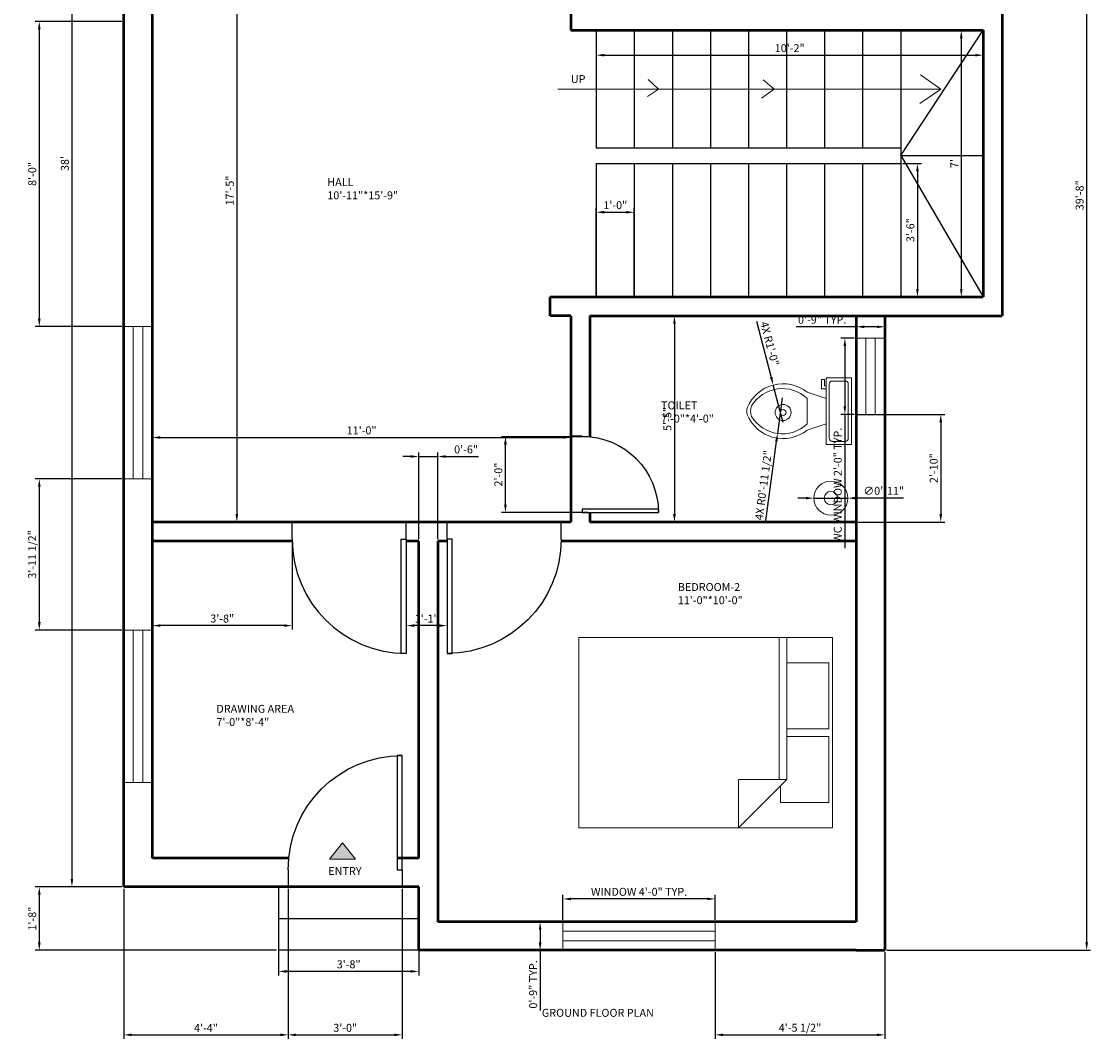
# Model space of a CAD drawing. Units: inches. Extents: x 1994 to 2331, y 1752 to 2286.
# Tile 1 of 2: x 1994 to 2331, y 1752 to 2073. Entities that reach past the tile are written whole.
import ezdxf

# ---------------------------------------------------------------- set-up
doc = ezdxf.new("R2010")
doc.units = ezdxf.units.IN
for name, color, linetype, lineweight in [('A-ANNO-DIMS', 2, 'Continuous', 18), ('A-ANNO-PATT', 7, 'Continuous', 18), ('A-ANNO-SYMB', 7, 'Continuous', 18), ('A-ANNO-TEXT', 7, 'Continuous', 25), ('A-AREA-IDEN', 7, 'Continuous', 25), ('A-DOOR', 3, 'Continuous', 25), ('A-FLOR-FIXT', 8, 'Continuous', 18), ('A-FLOR-STRS', 7, 'Continuous', 25), ('A-FURN', 9, 'Continuous', 18), ('A-GLAZ', 4, 'Continuous', 18), ('A-WALL', 7, 'Continuous', 50)]:
    doc.layers.add(name, color=color, linetype=linetype, lineweight=lineweight)
doc.styles.get("Standard").update_dxf_attribs({"font": 'arial.ttf'})
doc.dimstyles.new('ISO-25', dxfattribs={"dimtxt": 2.5, "dimasz": 2.5, "dimexe": 1.25, "dimexo": 0.625, "dimtad": 1, "dimdec": 1, "dimlunit": 3, "dimtxsty": 'Standard', "dimcen": 2.5, "dimadec": 0, "dimazin": 0, "dimtfac": 1, "dimtdec": 1, "dimtmove": 0, "dimatfit": 3, "dimfxl": 1, "dimarcsym": 0})

# ---------------------------------------------------------------- blocks, each defined once
blk = doc.blocks.new('*U2')
for p, q in [((0, 0), (0, -6)), ((40, 0), (40, -6))]:
    blk.add_line(p, q)
blk.add_lwpolyline([(0, 0), (0, 40), (1.75, 40), (1.75, 0)], close=True)
blk.add_arc((0, 0), 40, 0, 90)
blk = doc.blocks.new('Bed - Queen')
for p, q in [((0, -80.00003), (0, 0)), ((0, 0), (59.99999, 0)), ((59.99999, 0), (59.99999, -80.00003)), ((7.99999, -1.2), (28.79998, -1.2)), ((7.99999, -14.4), (7.99999, -1.2)), ((28.79998, -1.2), (28.79998, -14.4)), ((31.19999, -1.2), (51.99999, -1.2)), ((31.19999, -14.4), (31.19999, -1.2)), ((51.99999, -1.2), (51.99999, -16.4)), ((0, -14.4), (44.8, -14.4)), ((44.8, -16.8), (0, -16.8)), ((59.99999, -29.6), (44.8, -14.4)), ((44.8, -14.4), (44.8, -29.6)), ((51.99999, -16.4), (46.79936, -16.4)), ((44.8, -29.6), (59.99999, -29.6)), ((59.99999, -80.00003), (0, -80.00003))]:
    blk.add_line(p, q)
blk = doc.blocks.new('Toilet - top')
for p, q in [((9.5, -6), (9.5, -2)), ((-10, -8.5), (-8, -8.5)), ((-10, -9.5), (-10, -8.5)), ((-7, -9.5), (-10, -9.5)), ((-8, -8.5), (-8, -8)), ((-7, -8), (-7, -9.5)), ((-4, -8), (-6, -14)), ((4, -8), (6, -14)), ((4, -14), (-4, -14))]:
    blk.add_line(p, q)
blk.add_lwpolyline([(10.5, -8), (10.5, 0), (-10.5, 0), (-10.5, -8)], close=True)
for points in [[(-9.5, -2), (-9.5, -6)], [(8.5, -1), (-8.5, -1)], [(-8.5, -7), (8.5, -7)]]:
    blk.add_lwpolyline(points)
for centre, radius, start, end in [((-8.62, -1.88), 0.884, 81.8699, 188.1301), ((8.62, -1.88), 0.884, 351.8699, 98.1301), ((-8.62, -6.12), 0.884, 171.8699, 278.1301), ((8.62, -6.12), 0.884, 261.8699, 8.1301), ((3.52, -21.58), 12.17, 141.4691, 247.9714), ((4.2, -21.82), 11.33, 136.3677, 238.9468), ((-3.52, -21.58), 12.17, 292.0284, 38.5307), ((-4.2, -21.82), 11.33, 301.053, 43.6321), ((0, -27.88), 4, 245.7318, 294.2682), ((0, -29), 4, 254.8605, 285.1395)]:
    blk.add_arc(centre, radius, start, end)
blk = doc.blocks.new('*D7')
at = {"layer": 'A-ANNO-DIMS', "color": 0, "lineweight": -2, "transparency": 16777216}
for p, q in [((2025.95, 2256.2), (2008.97, 2256.2)), ((2010.22, 2253.7), (2010.22, 1802.7)), ((2025.95, 1800.2), (2008.97, 1800.2))]:
    blk.add_line(p, q, dxfattribs=at)
at = {"layer": 'A-ANNO-DIMS', "color": 0, "transparency": 16777216}
for points in [[(2009.8, 2253.7), (2010.63, 2253.7), (2010.22, 2256.2)], [(2009.8, 1802.7), (2010.63, 1802.7), (2010.22, 1800.2)]]:
    blk.add_solid(points, dxfattribs=at)
at = {"layer": 'Defpoints', "color": 0, "transparency": 16777216}
for p in [(2026.58, 2256.2), (2010.22, 1800.2), (2026.58, 1800.2)]:
    blk.add_point(p, dxfattribs=at)
at = {"layer": 'A-ANNO-DIMS', "color": 0, "transparency": 16777216, "insert": (2008.31, 2028.2), "char_height": 2.5, "attachment_point": 5, "rotation": 90}
blk.add_mtext("38'", dxfattribs=at)
blk = doc.blocks.new('*D9')
at = {"layer": 'A-ANNO-DIMS', "color": 0, "lineweight": -2, "transparency": 16777216}
for p, q in [((2296.95, 2070.2), (2289.44, 2070.2)), ((2290.69, 2067.7), (2290.69, 1988.7)), ((2296.95, 1986.2), (2289.44, 1986.2))]:
    blk.add_line(p, q, dxfattribs=at)
at = {"layer": 'A-ANNO-DIMS', "color": 0, "transparency": 16777216}
for points in [[(2290.28, 2067.7), (2291.11, 2067.7), (2290.69, 2070.2)], [(2290.28, 1988.7), (2291.11, 1988.7), (2290.69, 1986.2)]]:
    blk.add_solid(points, dxfattribs=at)
at = {"layer": 'Defpoints', "color": 0, "transparency": 16777216}
for p in [(2297.58, 2070.2), (2290.69, 1986.2), (2297.58, 1986.2)]:
    blk.add_point(p, dxfattribs=at)
at = {"layer": 'A-ANNO-DIMS', "color": 0, "transparency": 16777216, "insert": (2288.82, 2028.2), "char_height": 2.5, "attachment_point": 5, "rotation": 90}
blk.add_mtext("7'", dxfattribs=at)
blk = doc.blocks.new('*D10')
at = {"layer": 'A-ANNO-DIMS', "color": 0, "lineweight": -2, "transparency": 16777216}
for p, q in [((2272.2, 2028.2), (2278.11, 2028.2)), ((2276.86, 2025.7), (2276.86, 1988.7)), ((2272.2, 1986.2), (2278.11, 1986.2))]:
    blk.add_line(p, q, dxfattribs=at)
at = {"layer": 'A-ANNO-DIMS', "color": 0, "transparency": 16777216}
for points in [[(2276.44, 2025.7), (2277.28, 2025.7), (2276.86, 2028.2)], [(2276.44, 1988.7), (2277.28, 1988.7), (2276.86, 1986.2)]]:
    blk.add_solid(points, dxfattribs=at)
at = {"layer": 'Defpoints', "color": 0, "transparency": 16777216}
for p in [(2271.58, 2028.2), (2271.58, 1986.2), (2276.86, 1986.2)]:
    blk.add_point(p, dxfattribs=at)
at = {"layer": 'A-ANNO-DIMS', "color": 0, "transparency": 16777216, "insert": (2274.96, 2007.2), "char_height": 2.5, "attachment_point": 5, "rotation": 90}
blk.add_mtext('3\'-6"', dxfattribs=at)
blk = doc.blocks.new('*D11')
at = {"layer": 'A-ANNO-DIMS', "color": 0, "lineweight": -2, "transparency": 16777216}
for p, q in [((2175.58, 2069.58), (2175.58, 2061.11)), ((2297.58, 2069.58), (2297.58, 2061.11)), ((2178.08, 2062.36), (2295.08, 2062.36))]:
    blk.add_line(p, q, dxfattribs=at)
at = {"layer": 'A-ANNO-DIMS', "color": 0, "transparency": 16777216}
for points in [[(2178.08, 2062.78), (2178.08, 2061.95), (2175.58, 2062.36)], [(2295.08, 2062.78), (2295.08, 2061.95), (2297.58, 2062.36)]]:
    blk.add_solid(points, dxfattribs=at)
at = {"layer": 'Defpoints', "color": 0, "transparency": 16777216}
for p in [(2175.58, 2070.2), (2297.58, 2070.2), (2297.58, 2062.36)]:
    blk.add_point(p, dxfattribs=at)
at = {"layer": 'A-ANNO-DIMS', "color": 0, "transparency": 16777216, "insert": (2236.58, 2064.26), "char_height": 2.5, "attachment_point": 5}
blk.add_mtext('10\'-2"', dxfattribs=at)
blk = doc.blocks.new('WIN-48IN')
for p, q in [((0, 9), (48, 9)), ((0, 0), (0, 9)), ((48, 9), (48, 0)), ((0, 6), (48, 6)), ((48, 3), (0, 3)), ((48, 0), (0, 0))]:
    blk.add_line(p, q)
blk = doc.blocks.new('WIN-24IN')
for p, q in [((0, 0), (0, 24)), ((0, 24), (9, 24)), ((3, 0), (3, 24)), ((6, 24), (6, 0)), ((9, 24), (9, 0)), ((9, 0), (0, 0))]:
    blk.add_line(p, q)
blk = doc.blocks.new('*D14')
at = {"layer": 'A-ANNO-DIMS', "color": 0, "lineweight": -2, "transparency": 16777216}
for p, q in [((2165.08, 1789.83), (2165.08, 1797.65)), ((2213.08, 1789.83), (2213.08, 1797.65)), ((2210.58, 1796.4), (2167.58, 1796.4))]:
    blk.add_line(p, q, dxfattribs=at)
at = {"layer": 'A-ANNO-DIMS', "color": 0, "transparency": 16777216}
for points in [[(2167.58, 1796.82), (2167.58, 1795.99), (2165.08, 1796.4)], [(2210.58, 1796.82), (2210.58, 1795.99), (2213.08, 1796.4)]]:
    blk.add_solid(points, dxfattribs=at)
at = {"layer": 'Defpoints', "color": 0, "transparency": 16777216}
for p in [(2165.08, 1796.4), (2165.08, 1789.2), (2213.08, 1789.2)]:
    blk.add_point(p, dxfattribs=at)
at = {"layer": 'A-ANNO-DIMS', "color": 0, "transparency": 16777216, "insert": (2189.08, 1798.32), "char_height": 2.5, "attachment_point": 5}
blk.add_mtext('WINDOW 4\'-0" TYP.', dxfattribs=at)
blk = doc.blocks.new('*D15')
at = {"layer": 'A-ANNO-DIMS', "color": 0, "lineweight": -2, "transparency": 16777216}
for p, q in [((2164.46, 1789.2), (2156.63, 1789.2)), ((2157.88, 1786.7), (2157.88, 1782.7)), ((2164.46, 1780.2), (2156.63, 1780.2)), ((2157.88, 1780.2), (2157.88, 1761.22))]:
    blk.add_line(p, q, dxfattribs=at)
at = {"layer": 'A-ANNO-DIMS', "color": 0, "transparency": 16777216}
for points in [[(2157.46, 1786.7), (2158.3, 1786.7), (2157.88, 1789.2)], [(2157.46, 1782.7), (2158.3, 1782.7), (2157.88, 1780.2)]]:
    blk.add_solid(points, dxfattribs=at)
at = {"layer": 'Defpoints', "color": 0, "transparency": 16777216}
for p in [(2165.08, 1789.2), (2157.88, 1780.2), (2165.08, 1780.2)]:
    blk.add_point(p, dxfattribs=at)
at = {"layer": 'A-ANNO-DIMS', "color": 0, "transparency": 16777216, "insert": (2155.98, 1769.46), "char_height": 2.5, "attachment_point": 5, "rotation": 90}
blk.add_mtext('0\'-9" TYP.', dxfattribs=at)
blk = doc.blocks.new('*D16')
at = {"layer": 'A-ANNO-DIMS', "color": 0, "lineweight": -2, "transparency": 16777216}
for p, q in [((2256.95, 1973.15), (2252.73, 1973.15)), ((2253.98, 1970.65), (2253.98, 1951.65)), ((2256.95, 1949.15), (2252.73, 1949.15)), ((2253.98, 1949.15), (2253.98, 1906.97))]:
    blk.add_line(p, q, dxfattribs=at)
at = {"layer": 'A-ANNO-DIMS', "color": 0, "transparency": 16777216}
for points in [[(2253.56, 1970.65), (2254.4, 1970.65), (2253.98, 1973.15)], [(2253.56, 1951.65), (2254.4, 1951.65), (2253.98, 1949.15)]]:
    blk.add_solid(points, dxfattribs=at)
at = {"layer": 'Defpoints', "color": 0, "transparency": 16777216}
for p in [(2257.58, 1973.15), (2253.98, 1949.15), (2257.58, 1949.15)]:
    blk.add_point(p, dxfattribs=at)
at = {"layer": 'A-ANNO-DIMS', "color": 0, "transparency": 16777216, "insert": (2252.06, 1926.81), "char_height": 2.5, "attachment_point": 5, "rotation": 90}
blk.add_mtext('WC WINDOW 2\'-0" TYP.', dxfattribs=at)
blk = doc.blocks.new('*D17')
at = {"layer": 'A-ANNO-DIMS', "color": 0, "lineweight": -2, "transparency": 16777216}
for p, q in [((2257.58, 1976.75), (2238.59, 1976.75)), ((2257.58, 1973.77), (2257.58, 1978)), ((2264.08, 1976.75), (2260.08, 1976.75)), ((2266.58, 1973.77), (2266.58, 1978))]:
    blk.add_line(p, q, dxfattribs=at)
at = {"layer": 'A-ANNO-DIMS', "color": 0, "transparency": 16777216}
for points in [[(2260.08, 1977.16), (2260.08, 1976.33), (2257.58, 1976.75)], [(2264.08, 1977.16), (2264.08, 1976.33), (2266.58, 1976.75)]]:
    blk.add_solid(points, dxfattribs=at)
at = {"layer": 'Defpoints', "color": 0, "transparency": 16777216}
for p in [(2257.58, 1976.75), (2257.58, 1973.15), (2266.58, 1973.15)]:
    blk.add_point(p, dxfattribs=at)
at = {"layer": 'A-ANNO-DIMS', "color": 0, "transparency": 16777216, "insert": (2246.83, 1978.65), "char_height": 2.5, "attachment_point": 5}
blk.add_mtext('0\'-9" TYP.', dxfattribs=at)
blk = doc.blocks.new('*D24')
at = {"layer": 'A-ANNO-DIMS', "color": 0, "lineweight": -2, "transparency": 16777216}
for p, q in [((2267.2, 2256.2), (2331.48, 2256.2)), ((2330.23, 2253.7), (2330.23, 1782.7)), ((2267.2, 1780.2), (2331.48, 1780.2))]:
    blk.add_line(p, q, dxfattribs=at)
at = {"layer": 'A-ANNO-DIMS', "color": 0, "transparency": 16777216}
for points in [[(2329.81, 2253.7), (2330.65, 2253.7), (2330.23, 2256.2)], [(2329.81, 1782.7), (2330.65, 1782.7), (2330.23, 1780.2)]]:
    blk.add_solid(points, dxfattribs=at)
at = {"layer": 'Defpoints', "color": 0, "transparency": 16777216}
for p in [(2266.58, 2256.2), (2266.58, 1780.2), (2330.23, 1780.2)]:
    blk.add_point(p, dxfattribs=at)
at = {"layer": 'A-ANNO-DIMS', "color": 0, "transparency": 16777216, "insert": (2328.33, 2018.2), "char_height": 2.5, "attachment_point": 5, "rotation": 90}
blk.add_mtext('39\'-8"', dxfattribs=at)
blk = doc.blocks.new('*D26')
at = {"layer": 'A-ANNO-DIMS', "color": 0, "lineweight": -2, "transparency": 16777216}
for p, q in [((2025.95, 1800.2), (1998.68, 1800.2)), ((1999.93, 1797.7), (1999.93, 1782.7)), ((2074.77, 1780.2), (1998.68, 1780.2))]:
    blk.add_line(p, q, dxfattribs=at)
at = {"layer": 'A-ANNO-DIMS', "color": 0, "transparency": 16777216}
for points in [[(1999.51, 1797.7), (2000.35, 1797.7), (1999.93, 1800.2)], [(1999.51, 1782.7), (2000.35, 1782.7), (1999.93, 1780.2)]]:
    blk.add_solid(points, dxfattribs=at)
at = {"layer": 'Defpoints', "color": 0, "transparency": 16777216}
for p in [(2026.58, 1800.2), (1999.93, 1780.2), (2075.4, 1780.2)]:
    blk.add_point(p, dxfattribs=at)
at = {"layer": 'A-ANNO-DIMS', "color": 0, "transparency": 16777216, "insert": (1998.03, 1790.2), "char_height": 2.5, "attachment_point": 5, "rotation": 90}
blk.add_mtext('1\'-8"', dxfattribs=at)
blk = doc.blocks.new('*D30')
at = {"layer": 'A-ANNO-DIMS', "color": 0, "lineweight": -2, "transparency": 16777216}
for p, q in [((2025.95, 2073.01), (1998.68, 2073.01)), ((1999.93, 2070.51), (1999.93, 1979.32)), ((2025.95, 1976.82), (1998.68, 1976.82))]:
    blk.add_line(p, q, dxfattribs=at)
at = {"layer": 'A-ANNO-DIMS', "color": 0, "transparency": 16777216}
for points in [[(1999.51, 2070.51), (2000.35, 2070.51), (1999.93, 2073.01)], [(1999.51, 1979.32), (2000.35, 1979.32), (1999.93, 1976.82)]]:
    blk.add_solid(points, dxfattribs=at)
at = {"layer": 'Defpoints', "color": 0, "transparency": 16777216}
for p in [(2026.58, 2073.01), (1999.93, 1976.82), (2026.58, 1976.82)]:
    blk.add_point(p, dxfattribs=at)
at = {"layer": 'A-ANNO-DIMS', "color": 0, "transparency": 16777216, "insert": (1998.03, 2024.91), "char_height": 2.5, "attachment_point": 5, "rotation": 90}
blk.add_mtext('8\'-0"', dxfattribs=at)
blk = doc.blocks.new('*D31')
at = {"layer": 'A-ANNO-DIMS', "color": 0, "lineweight": -2, "transparency": 16777216}
for p, q in [((2025.95, 1928.82), (1998.68, 1928.82)), ((1999.93, 1926.32), (1999.93, 1883.65)), ((2025.95, 1881.15), (1998.68, 1881.15))]:
    blk.add_line(p, q, dxfattribs=at)
at = {"layer": 'A-ANNO-DIMS', "color": 0, "transparency": 16777216}
for points in [[(1999.51, 1926.32), (2000.35, 1926.32), (1999.93, 1928.82)], [(1999.51, 1883.65), (2000.35, 1883.65), (1999.93, 1881.15)]]:
    blk.add_solid(points, dxfattribs=at)
at = {"layer": 'Defpoints', "color": 0, "transparency": 16777216}
for p in [(2026.58, 1928.82), (1999.93, 1881.15), (2026.58, 1881.15)]:
    blk.add_point(p, dxfattribs=at)
at = {"layer": 'A-ANNO-DIMS', "color": 0, "transparency": 16777216, "insert": (1998.01, 1904.99), "char_height": 2.5, "attachment_point": 5, "rotation": 90}
blk.add_mtext('3\'-11 1/2"', dxfattribs=at)
blk = doc.blocks.new('*D34')
at = {"layer": 'A-ANNO-DIMS', "color": 0, "lineweight": -2, "transparency": 16777216}
for p, q in [((2258.2, 1949.15), (2285.48, 1949.15)), ((2284.23, 1946.65), (2284.23, 1917.7)), ((2258.2, 1915.2), (2285.48, 1915.2))]:
    blk.add_line(p, q, dxfattribs=at)
at = {"layer": 'A-ANNO-DIMS', "color": 0, "transparency": 16777216}
for points in [[(2283.81, 1946.65), (2284.65, 1946.65), (2284.23, 1949.15)], [(2283.81, 1917.7), (2284.65, 1917.7), (2284.23, 1915.2)]]:
    blk.add_solid(points, dxfattribs=at)
at = {"layer": 'Defpoints', "color": 0, "transparency": 16777216}
for p in [(2257.58, 1949.15), (2257.58, 1915.2), (2284.23, 1915.2)]:
    blk.add_point(p, dxfattribs=at)
at = {"layer": 'A-ANNO-DIMS', "color": 0, "transparency": 16777216, "insert": (2282.33, 1932.18), "char_height": 2.5, "attachment_point": 5, "rotation": 90}
blk.add_mtext('2\'-10"', dxfattribs=at)
blk = doc.blocks.new('*D35')
at = {"layer": 'A-ANNO-DIMS', "color": 0, "lineweight": -2, "transparency": 16777216}
for p, q in [((2213.08, 1779.58), (2213.08, 1752.3)), ((2266.58, 1779.58), (2266.58, 1752.3)), ((2215.58, 1753.55), (2264.08, 1753.55))]:
    blk.add_line(p, q, dxfattribs=at)
at = {"layer": 'A-ANNO-DIMS', "color": 0, "transparency": 16777216}
for points in [[(2215.58, 1753.97), (2215.58, 1753.14), (2213.08, 1753.55)], [(2264.08, 1753.97), (2264.08, 1753.14), (2266.58, 1753.55)]]:
    blk.add_solid(points, dxfattribs=at)
at = {"layer": 'Defpoints', "color": 0, "transparency": 16777216}
for p in [(2213.08, 1780.2), (2266.58, 1780.2), (2266.58, 1753.55)]:
    blk.add_point(p, dxfattribs=at)
at = {"layer": 'A-ANNO-DIMS', "color": 0, "transparency": 16777216, "insert": (2239.83, 1755.47), "char_height": 2.5, "attachment_point": 5}
blk.add_mtext('4\'-5 1/2"', dxfattribs=at)
blk = doc.blocks.new('*D36')
at = {"layer": 'A-ANNO-DIMS', "color": 0, "lineweight": -2, "transparency": 16777216}
for p, q in [((2174.2, 1980.2), (2201.48, 1980.2)), ((2200.23, 1977.7), (2200.23, 1917.7)), ((2174.2, 1915.2), (2201.48, 1915.2))]:
    blk.add_line(p, q, dxfattribs=at)
at = {"layer": 'A-ANNO-DIMS', "color": 0, "transparency": 16777216}
for points in [[(2199.81, 1977.7), (2200.65, 1977.7), (2200.23, 1980.2)], [(2199.81, 1917.7), (2200.65, 1917.7), (2200.23, 1915.2)]]:
    blk.add_solid(points, dxfattribs=at)
at = {"layer": 'Defpoints', "color": 0, "transparency": 16777216}
for p in [(2173.58, 1980.2), (2173.58, 1915.2), (2200.23, 1915.2)]:
    blk.add_point(p, dxfattribs=at)
at = {"layer": 'A-ANNO-DIMS', "color": 0, "transparency": 16777216, "insert": (2198.33, 1947.7), "char_height": 2.5, "attachment_point": 5, "rotation": 90}
blk.add_mtext('5\'-5"', dxfattribs=at)
blk = doc.blocks.new('*D37')
at = {"layer": 'A-ANNO-DIMS', "color": 0, "lineweight": -2, "transparency": 16777216}
for p, q in [((2175.58, 1986.83), (2175.58, 2014.1)), ((2187.58, 1986.83), (2187.58, 2014.1)), ((2178.08, 2012.85), (2185.08, 2012.85))]:
    blk.add_line(p, q, dxfattribs=at)
at = {"layer": 'A-ANNO-DIMS', "color": 0, "transparency": 16777216}
for points in [[(2178.08, 2013.27), (2178.08, 2012.44), (2175.58, 2012.85)], [(2185.08, 2013.27), (2185.08, 2012.44), (2187.58, 2012.85)]]:
    blk.add_solid(points, dxfattribs=at)
at = {"layer": 'Defpoints', "color": 0, "transparency": 16777216}
for p in [(2187.58, 2012.85), (2175.58, 1986.2), (2187.58, 1986.2)]:
    blk.add_point(p, dxfattribs=at)
at = {"layer": 'A-ANNO-DIMS', "color": 0, "transparency": 16777216, "insert": (2181.58, 2014.76), "char_height": 2.5, "attachment_point": 5}
blk.add_mtext('1\'-0"', dxfattribs=at)
blk = doc.blocks.new('*D38')
at = {"layer": 'A-ANNO-DIMS', "color": 0, "lineweight": -2, "transparency": 16777216}
for p, q in [((2117.08, 1935.85), (2114.58, 1935.85)), ((2119.58, 1909.83), (2119.58, 1937.1)), ((2119.58, 1935.85), (2125.58, 1935.85)), ((2125.58, 1909.83), (2125.58, 1937.1)), ((2128.08, 1935.85), (2138.47, 1935.85))]:
    blk.add_line(p, q, dxfattribs=at)
at = {"layer": 'A-ANNO-DIMS', "color": 0, "transparency": 16777216}
for points in [[(2117.08, 1936.27), (2117.08, 1935.44), (2119.58, 1935.85)], [(2128.08, 1936.27), (2128.08, 1935.44), (2125.58, 1935.85)]]:
    blk.add_solid(points, dxfattribs=at)
at = {"layer": 'Defpoints', "color": 0, "transparency": 16777216}
for p in [(2125.58, 1935.85), (2119.58, 1909.2), (2125.58, 1909.2)]:
    blk.add_point(p, dxfattribs=at)
at = {"layer": 'A-ANNO-DIMS', "color": 0, "transparency": 16777216, "insert": (2134.53, 1937.76), "char_height": 2.5, "attachment_point": 5}
blk.add_mtext('0\'-6"', dxfattribs=at)
blk = doc.blocks.new('*D39')
at = {"layer": 'A-ANNO-DIMS', "color": 0, "lineweight": -2, "transparency": 16777216}
for p, q in [((2026.58, 1799.58), (2026.58, 1752.3)), ((2078.4, 1799.58), (2078.4, 1752.3)), ((2029.08, 1753.55), (2075.9, 1753.55))]:
    blk.add_line(p, q, dxfattribs=at)
at = {"layer": 'A-ANNO-DIMS', "color": 0, "transparency": 16777216}
for points in [[(2029.08, 1753.97), (2029.08, 1753.14), (2026.58, 1753.55)], [(2075.9, 1753.97), (2075.9, 1753.14), (2078.4, 1753.55)]]:
    blk.add_solid(points, dxfattribs=at)
at = {"layer": 'Defpoints', "color": 0, "transparency": 16777216}
for p in [(2026.58, 1800.2), (2078.4, 1800.2), (2078.4, 1753.55)]:
    blk.add_point(p, dxfattribs=at)
at = {"layer": 'A-ANNO-DIMS', "color": 0, "transparency": 16777216, "insert": (2052.49, 1755.43), "char_height": 2.5, "attachment_point": 5}
blk.add_mtext('4\'-4"', dxfattribs=at)
blk = doc.blocks.new('*D40')
at = {"layer": 'A-ANNO-DIMS', "color": 0, "lineweight": -2, "transparency": 16777216}
for p, q in [((2036.2, 2124.2), (2063.48, 2124.2)), ((2062.23, 2121.7), (2062.23, 1917.7)), ((2036.2, 1915.2), (2063.48, 1915.2))]:
    blk.add_line(p, q, dxfattribs=at)
at = {"layer": 'A-ANNO-DIMS', "color": 0, "transparency": 16777216}
for points in [[(2061.81, 2121.7), (2062.65, 2121.7), (2062.23, 2124.2)], [(2061.81, 1917.7), (2062.65, 1917.7), (2062.23, 1915.2)]]:
    blk.add_solid(points, dxfattribs=at)
at = {"layer": 'Defpoints', "color": 0, "transparency": 16777216}
for p in [(2035.58, 2124.2), (2035.58, 1915.2), (2062.23, 1915.2)]:
    blk.add_point(p, dxfattribs=at)
at = {"layer": 'A-ANNO-DIMS', "color": 0, "transparency": 16777216, "insert": (2060.33, 2019.7), "char_height": 2.5, "attachment_point": 5, "rotation": 90}
blk.add_mtext('17\'-5"', dxfattribs=at)
blk = doc.blocks.new('*D41')
at = {"layer": 'A-ANNO-DIMS', "color": 0, "lineweight": -2, "transparency": 16777216}
for p, q in [((2035.58, 1915.83), (2035.58, 1943.1)), ((2167.58, 1915.83), (2167.58, 1943.1)), ((2038.08, 1941.85), (2165.08, 1941.85))]:
    blk.add_line(p, q, dxfattribs=at)
at = {"layer": 'A-ANNO-DIMS', "color": 0, "transparency": 16777216}
for points in [[(2038.08, 1942.27), (2038.08, 1941.44), (2035.58, 1941.85)], [(2165.08, 1942.27), (2165.08, 1941.44), (2167.58, 1941.85)]]:
    blk.add_solid(points, dxfattribs=at)
at = {"layer": 'Defpoints', "color": 0, "transparency": 16777216}
for p in [(2167.58, 1941.85), (2035.58, 1915.2), (2167.58, 1915.2)]:
    blk.add_point(p, dxfattribs=at)
at = {"layer": 'A-ANNO-DIMS', "color": 0, "transparency": 16777216, "insert": (2101.58, 1943.76), "char_height": 2.5, "attachment_point": 5}
blk.add_mtext('11\'-0"', dxfattribs=at)
blk = doc.blocks.new('*D42')
at = {"layer": 'A-ANNO-DIMS', "color": 0, "lineweight": -2, "transparency": 16777216}
for p, q in [((2078.4, 1799.58), (2078.4, 1752.3)), ((2114.4, 1799.58), (2114.4, 1752.3)), ((2080.9, 1753.55), (2111.9, 1753.55))]:
    blk.add_line(p, q, dxfattribs=at)
at = {"layer": 'A-ANNO-DIMS', "color": 0, "transparency": 16777216}
for points in [[(2080.9, 1753.97), (2080.9, 1753.14), (2078.4, 1753.55)], [(2111.9, 1753.97), (2111.9, 1753.14), (2114.4, 1753.55)]]:
    blk.add_solid(points, dxfattribs=at)
at = {"layer": 'Defpoints', "color": 0, "transparency": 16777216}
for p in [(2078.4, 1800.2), (2114.4, 1800.2), (2114.4, 1753.55)]:
    blk.add_point(p, dxfattribs=at)
at = {"layer": 'A-ANNO-DIMS', "color": 0, "transparency": 16777216, "insert": (2096.4, 1755.46), "char_height": 2.5, "attachment_point": 5}
blk.add_mtext('3\'-0"', dxfattribs=at)
blk = doc.blocks.new('*D46')
at = {"layer": 'A-ANNO-DIMS', "color": 0, "lineweight": -2, "transparency": 16777216}
for p, q in [((2075.4, 1799.58), (2075.4, 1772.3)), ((2119.58, 1799.58), (2119.58, 1772.3)), ((2117.08, 1773.55), (2077.9, 1773.55))]:
    blk.add_line(p, q, dxfattribs=at)
at = {"layer": 'A-ANNO-DIMS', "color": 0, "transparency": 16777216}
for points in [[(2077.9, 1773.97), (2077.9, 1773.14), (2075.4, 1773.55)], [(2117.08, 1773.97), (2117.08, 1773.14), (2119.58, 1773.55)]]:
    blk.add_solid(points, dxfattribs=at)
at = {"layer": 'Defpoints', "color": 0, "transparency": 16777216}
for p in [(2075.4, 1800.2), (2119.58, 1800.2), (2075.4, 1773.55)]:
    blk.add_point(p, dxfattribs=at)
at = {"layer": 'A-ANNO-DIMS', "color": 0, "transparency": 16777216, "insert": (2097.49, 1775.46), "char_height": 2.5, "attachment_point": 5}
blk.add_mtext('3\'-8"', dxfattribs=at)
blk = doc.blocks.new('*D47')
at = {"layer": 'A-ANNO-DIMS', "color": 0, "lineweight": -2, "transparency": 16777216}
for p, q in [((2035.58, 1908.58), (2035.58, 1881.3)), ((2079.66, 1908.58), (2079.66, 1881.3)), ((2077.16, 1882.55), (2038.08, 1882.55))]:
    blk.add_line(p, q, dxfattribs=at)
at = {"layer": 'A-ANNO-DIMS', "color": 0, "transparency": 16777216}
for points in [[(2038.08, 1882.97), (2038.08, 1882.14), (2035.58, 1882.55)], [(2077.16, 1882.97), (2077.16, 1882.14), (2079.66, 1882.55)]]:
    blk.add_solid(points, dxfattribs=at)
at = {"layer": 'Defpoints', "color": 0, "transparency": 16777216}
for p in [(2035.58, 1909.2), (2079.66, 1909.2), (2035.58, 1882.55)]:
    blk.add_point(p, dxfattribs=at)
at = {"layer": 'A-ANNO-DIMS', "color": 0, "transparency": 16777216, "insert": (2057.62, 1884.46), "char_height": 2.5, "attachment_point": 5}
blk.add_mtext('3\'-8"', dxfattribs=at)
blk = doc.blocks.new('*D48')
at = {"layer": 'A-ANNO-DIMS', "color": 0, "lineweight": -2, "transparency": 16777216}
for p, q in [((2115.66, 1908.58), (2115.66, 1881.3)), ((2128.52, 1908.58), (2128.52, 1881.3)), ((2126.02, 1882.55), (2118.16, 1882.55))]:
    blk.add_line(p, q, dxfattribs=at)
at = {"layer": 'A-ANNO-DIMS', "color": 0, "transparency": 16777216}
for points in [[(2118.16, 1882.97), (2118.16, 1882.14), (2115.66, 1882.55)], [(2126.02, 1882.97), (2126.02, 1882.14), (2128.52, 1882.55)]]:
    blk.add_solid(points, dxfattribs=at)
at = {"layer": 'Defpoints', "color": 0, "transparency": 16777216}
for p in [(2115.66, 1909.2), (2128.52, 1909.2), (2115.66, 1882.55)]:
    blk.add_point(p, dxfattribs=at)
at = {"layer": 'A-ANNO-DIMS', "color": 0, "transparency": 16777216, "insert": (2122.09, 1884.43), "char_height": 2.5, "attachment_point": 5}
blk.add_mtext('1\'-1"', dxfattribs=at)
blk = doc.blocks.new('*D49')
at = {"layer": 'A-ANNO-DIMS', "color": 0, "lineweight": -2, "transparency": 16777216}
for p, q in [((2172.95, 1942.11), (2145.68, 1942.11)), ((2146.93, 1920.73), (2146.93, 1939.61)), ((2172.95, 1918.23), (2145.68, 1918.23))]:
    blk.add_line(p, q, dxfattribs=at)
at = {"layer": 'A-ANNO-DIMS', "color": 0, "transparency": 16777216}
for points in [[(2146.51, 1939.61), (2147.35, 1939.61), (2146.93, 1942.11)], [(2146.51, 1920.73), (2147.35, 1920.73), (2146.93, 1918.23)]]:
    blk.add_solid(points, dxfattribs=at)
at = {"layer": 'Defpoints', "color": 0, "transparency": 16777216}
for p in [(2146.93, 1942.11), (2173.58, 1942.11), (2173.58, 1918.23)]:
    blk.add_point(p, dxfattribs=at)
at = {"layer": 'A-ANNO-DIMS', "color": 0, "transparency": 16777216, "insert": (2145.03, 1930.17), "char_height": 2.5, "attachment_point": 5, "rotation": 90}
blk.add_mtext('2\'-0"', dxfattribs=at)
blk = doc.blocks.new('*D56')
at = {"layer": 'A-ANNO-DIMS', "color": 0, "lineweight": -2, "transparency": 16777216}
for p, q in [((2241.69, 1922.74), (2239.19, 1922.74)), ((2244.19, 1922.74), (2254.95, 1922.74)), ((2272.51, 1922.74), (2257.45, 1922.74))]:
    blk.add_line(p, q, dxfattribs=at)
at = {"layer": 'A-ANNO-DIMS', "color": 0, "transparency": 16777216}
for points in [[(2241.69, 1923.16), (2241.69, 1922.32), (2244.19, 1922.74)], [(2257.45, 1923.16), (2257.45, 1922.32), (2254.95, 1922.74)]]:
    blk.add_solid(points, dxfattribs=at)
at = {"layer": 'Defpoints', "color": 0, "transparency": 16777216}
for p in [(2244.19, 1922.74), (2254.95, 1922.74)]:
    blk.add_point(p, dxfattribs=at)
at = {"layer": 'A-ANNO-DIMS', "color": 0, "transparency": 16777216, "insert": (2266.23, 1924.71), "char_height": 2.5, "attachment_point": 5, "rotation": 0.0033}
blk.add_mtext('∅0\'-11"', dxfattribs=at)
blk = doc.blocks.new('*D58')
at = {"layer": 'A-ANNO-DIMS', "color": 0, "lineweight": -2, "transparency": 16777216}
for p, q in [((2226.12, 1978.47), (2230.76, 1960.81)), ((2234.49, 1946.63), (2231.39, 1958.39))]:
    blk.add_line(p, q, dxfattribs=at)
at = {"layer": 'A-ANNO-DIMS', "color": 0, "transparency": 16777216}
blk.add_solid([(2231.16, 1960.92), (2230.35, 1960.71), (2231.39, 1958.39)], dxfattribs=at)
at = {"layer": 'Defpoints', "color": 0, "transparency": 16777216}
for p in [(2231.39, 1958.39), (2234.49, 1946.63)]:
    blk.add_point(p, dxfattribs=at)
at = {"layer": 'A-ANNO-DIMS', "color": 0, "transparency": 16777216, "insert": (2229.96, 1971.34), "char_height": 2.5, "attachment_point": 5, "rotation": 284.7215}
blk.add_mtext('4X R1\'-0"', dxfattribs=at)
blk = doc.blocks.new('*D59')
at = {"layer": 'A-ANNO-DIMS', "color": 0, "lineweight": -2, "transparency": 16777216}
for p, q in [((2234.25, 1954.34), (2232.74, 1943.12)), ((2228.94, 1914.84), (2232.41, 1940.64))]:
    blk.add_line(p, q, dxfattribs=at)
at = {"layer": 'A-ANNO-DIMS', "color": 0, "transparency": 16777216}
blk.add_solid([(2231.99, 1940.69), (2232.82, 1940.58), (2232.74, 1943.12)], dxfattribs=at)
at = {"layer": 'Defpoints', "color": 0, "transparency": 16777216}
for p in [(2234.25, 1954.34), (2232.74, 1943.12)]:
    blk.add_point(p, dxfattribs=at)
at = {"layer": 'A-ANNO-DIMS', "color": 0, "transparency": 16777216, "insert": (2228.6, 1926.76), "char_height": 2.5, "attachment_point": 5, "rotation": 82.3428}
blk.add_mtext('4X R0\'-11 1/2"', dxfattribs=at)

msp = doc.modelspace()

# ---------------------------------------------------------------- hatches: boundary and pattern name
at = {"layer": 'A-ANNO-PATT'}
h = msp.add_hatch(color=256, dxfattribs=at)
h.dxf.hatch_style = 1
h.paths.add_polyline_path([(2095.55, 1814.06), (2091.5, 1808.98), (2099.61, 1808.98)])

# ---------------------------------------------------------------- linework, layer by layer
at = {"layer": 'A-ANNO-SYMB'}
for p, q in [((2191.95, 2054.71), (2195.21, 2051.7)), ((2228.18, 2054.64), (2231.65, 2051.7)), ((2284.24, 2051.7), (2277.78, 2056.15)), ((2163.51, 2051.7), (2284.24, 2051.7)), ((2195.21, 2051.7), (2191.74, 2049.3)), ((2231.65, 2051.7), (2227.7, 2048.82)), ((2284.24, 2051.7), (2277.6, 2047.16)), ((2095.55, 1814.06), (2091.5, 1808.98)), ((2099.61, 1808.98), (2095.55, 1814.06)), ((2091.5, 1808.98), (2099.61, 1808.98))]:
    msp.add_line(p, q, dxfattribs=at)
at = {"layer": 'A-FLOR-FIXT'}
for centre, radius in [((2234.49, 1949.74), 2.53), ((2234.49, 1949.74), 0.937), ((2249.57, 1922.74), 5.38), ((2249.57, 1922.74), 2.12)]:
    msp.add_circle(centre, radius, dxfattribs=at)
at = {"layer": 'A-FLOR-STRS'}
for p, q in [((2175.58, 2070.2), (2175.58, 2033.2)), ((2187.58, 2070.2), (2187.58, 2033.2)), ((2199.58, 2070.2), (2199.58, 2033.2)), ((2211.58, 2070.2), (2211.58, 2033.2)), ((2223.58, 2070.2), (2223.58, 2033.2)), ((2235.58, 2070.2), (2235.58, 2033.2)), ((2247.58, 2070.2), (2247.58, 2033.2)), ((2259.58, 2070.2), (2259.58, 2033.2)), ((2271.58, 2070.2), (2271.58, 1986.2)), ((2271.58, 2030.7), (2297.58, 2070.2)), ((2175.58, 2033.2), (2271.58, 2033.2)), ((2271.58, 2030.7), (2297.58, 2030.7)), ((2271.58, 2030.7), (2297.58, 1986.2)), ((2175.58, 2028.2), (2271.58, 2028.2)), ((2175.58, 2028.2), (2175.58, 1986.2)), ((2187.58, 2028.2), (2187.58, 1986.2)), ((2199.58, 2028.2), (2199.58, 1986.2)), ((2211.58, 2028.2), (2211.58, 1986.2)), ((2223.58, 2028.2), (2223.58, 1986.2)), ((2235.58, 2028.2), (2235.58, 1986.2)), ((2247.58, 2028.2), (2247.58, 1986.2)), ((2259.58, 2028.2), (2259.58, 1986.2)), ((2075.4, 1800.2), (2075.4, 1780.2)), ((2075.4, 1790.2), (2119.58, 1790.2)), ((2119.58, 1780.2), (2075.4, 1780.2))]:
    msp.add_line(p, q, dxfattribs=at)
at = {"layer": 'A-WALL'}
for p, q in [((2026.58, 1800.2), (2026.58, 2256.2)), ((2035.58, 1809.2), (2035.58, 2247.2)), ((2167.58, 2124.2), (2167.58, 2070.2)), ((2303.58, 2076.2), (2303.58, 1980.2)), ((2167.58, 2070.2), (2297.58, 2070.2)), ((2297.58, 2070.2), (2297.58, 1986.2)), ((2161.07, 1986.2), (2297.58, 1986.2)), ((2161.07, 1980.2), (2161.07, 1986.2)), ((2167.58, 1980.2), (2161.07, 1980.2)), ((2167.58, 1980.2), (2167.58, 1915.2)), ((2173.58, 1980.2), (2303.58, 1980.2)), ((2173.58, 1980.2), (2173.58, 1942.11)), ((2257.58, 1980.2), (2257.58, 1789.2)), ((2266.58, 1980.2), (2266.58, 1780.2)), ((2173.58, 1918.23), (2173.58, 1915.2)), ((2167.58, 1915.2), (2035.58, 1915.2)), ((2257.58, 1915.2), (2173.58, 1915.2)), ((2079.66, 1909.2), (2035.58, 1909.2)), ((2119.58, 1909.2), (2115.66, 1909.2)), ((2119.58, 1809.2), (2119.58, 1909.2)), ((2125.58, 1909.2), (2125.58, 1789.2)), ((2128.52, 1909.2), (2125.58, 1909.2)), ((2257.58, 1909.2), (2164.52, 1909.2)), ((2078.58, 1809.2), (2035.58, 1809.2)), ((2119.58, 1809.2), (2112.82, 1809.2)), ((2119.58, 1800.2), (2026.58, 1800.2)), ((2119.58, 1780.2), (2119.58, 1800.2)), ((2257.58, 1789.2), (2125.58, 1789.2)), ((2257.58, 1780.2), (2119.58, 1780.2)), ((2257.58, 1780.2), (2266.58, 1780.2))]:
    msp.add_line(p, q, dxfattribs=at)

# ---------------------------------------------------------------- block references
at = {"layer": 'A-DOOR'}
for p, xscale, yscale, zscale, rotation in [((2171.18, 1918.23), -0.5999999999999969, 0.5999999999999969, 0.5999999999999969, 270), ((2115.66, 1909.8), 0.8999999999998362, 0.8999999999998362, 0.8999999999998362, 180), ((2128.52, 1909.8), -0.8999999999998362, 0.8999999999998362, 0.8999999999998362, 180)]:
    msp.add_blockref('*U2', p, dxfattribs=dict(at, xscale=xscale, yscale=yscale, zscale=zscale, rotation=rotation))
at = {"layer": 'A-DOOR', "xscale": -0.8999999999998362, "yscale": 0.8999999999998362, "zscale": 0.8999999999998362}
msp.add_blockref('*U2', (2114.4, 1805.6), dxfattribs=at)
at = {"layer": 'A-FLOR-FIXT', "rotation": 270}
msp.add_blockref('Toilet - top', (2256.07, 1950.14), dxfattribs=at)
at = {"layer": 'A-FURN', "rotation": 270}
msp.add_blockref('Bed - Queen', (2250.08, 1878.82), dxfattribs=at)
at = {"layer": 'A-GLAZ'}
for name, p, rotation in [('WIN-48IN', (2026.58, 1976.82), 270.0000000000001), ('WIN-24IN', (2266.58, 1973.15), 180), ('WIN-48IN', (2026.58, 1881.15), 270), ('WIN-48IN', (2213.08, 1789.2), 180)]:
    msp.add_blockref(name, p, dxfattribs=dict(at, rotation=rotation))

# ---------------------------------------------------------------- texts
at = {"layer": 'A-ANNO-TEXT', "char_height": 2.5, "attachment_point": 1}
for s, width, insert in [('UP', 8.317, (2167.55, 2056.08)), ('ENTRY', 23.0635, (2091.07, 1806.44)), ('GROUND FLOOR PLAN', 187.3832, (2158.4, 1761.75))]:
    msp.add_mtext_dynamic_manual_height_columns(s, width=width, gutter_width=12.5, heights=[0], dxfattribs=dict(at, insert=insert))
at = {"layer": 'A-AREA-IDEN', "char_height": 2.5, "attachment_point": 1}
for s, width, insert in [('HALL\\P10\'-11"*15\'-9"', 89.9636, (2090.76, 2023.6)), ('TOILET\\P7\'-0"*4\'-0"', 43.6967, (2196.01, 1953.23)), ('BEDROOM-2\\P11\'-0"*10\'-0"', 65.5389, (2201.3, 1895.97)), ('DRAWING AREA\\P7\'-0"*8\'-4"', 51.3928, (2055.78, 1857.58))]:
    msp.add_mtext_dynamic_manual_height_columns(s, width=width, gutter_width=12.5, heights=[0], dxfattribs=dict(at, insert=insert))

# ---------------------------------------------------------------- dimensions: what is measured, and where the dimension line sits
at = {"layer": 'A-ANNO-DIMS'}
for base, p1, p2, angle, override, picture, middle in [((2010.22, 1800.2), (2026.58, 2256.2), (2026.58, 1800.2), 90, {"dimclrd": 0, "dimclre": 0, "dimclrt": 0}, '*D7', (2008.31, 2028.2)), ((2330.23, 1780.2), (2266.58, 2256.2), (2266.58, 1780.2), 90, {"dimdec": 1, "dimlfac": 1, "dimrnd": 0, "dimzin": 1, "dimdsep": 46, "dimlunit": 4, "dimfrac": 2}, '*D24', (2328.33, 2018.2)), ((2062.23, 1915.2), (2035.58, 2124.2), (2035.58, 1915.2), 270, {"dimdec": 1, "dimlfac": 1, "dimrnd": 0, "dimzin": 1, "dimdsep": 46, "dimlunit": 4, "dimfrac": 2}, '*D40', (2060.33, 2019.7)), ((1999.93, 1976.82), (2026.58, 2073.01), (2026.58, 1976.82), 90, {"dimdec": 1, "dimlfac": 1, "dimrnd": 0, "dimzin": 1, "dimdsep": 46, "dimlunit": 4, "dimfrac": 2}, '*D30', (1998.03, 2024.91)), ((2290.69, 1986.2), (2297.58, 2070.2), (2297.58, 1986.2), 90, {"dimclrd": 0, "dimclre": 0, "dimclrt": 0}, '*D9', (2288.82, 2028.2)), ((2276.86, 1986.2), (2271.58, 2028.2), (2271.58, 1986.2), 90, {"dimclrd": 0, "dimclre": 0, "dimclrt": 0}, '*D10', (2274.96, 2007.2)), ((2200.23, 1915.2), (2173.58, 1980.2), (2173.58, 1915.2), 270, {"dimdec": 1, "dimlfac": 1, "dimrnd": 0, "dimzin": 1, "dimdsep": 46, "dimlunit": 4, "dimfrac": 2}, '*D36', (2198.33, 1947.7)), ((2284.2293, 1915.2046), (2257.5793, 1949.1466), (2257.5793, 1915.2046), 270, {"dimdec": 1, "dimlfac": 1, "dimrnd": 0, "dimzin": 1, "dimdsep": 46, "dimlunit": 4, "dimfrac": 2}, '*D34', (2282.3279, 1932.1756)), ((2146.93, 1942.11), (2173.58, 1918.23), (2173.58, 1942.11), 90, {"dimdec": 1, "dimlfac": 1, "dimrnd": 0, "dimzin": 1, "dimdsep": 46, "dimlunit": 4, "dimfrac": 2}, '*D49', (2145.03, 1930.17)), ((1999.93, 1881.15), (2026.58, 1928.82), (2026.58, 1881.15), 90, {"dimdec": 1, "dimlfac": 1, "dimrnd": 0, "dimzin": 1, "dimdsep": 46, "dimlunit": 4, "dimfrac": 2}, '*D31', (1998.01, 1904.99)), ((2035.58, 1882.55), (2079.66, 1909.2), (2035.58, 1909.2), 180, {"dimdec": 1, "dimlfac": 1, "dimrnd": 0, "dimzin": 1, "dimdsep": 46, "dimlunit": 4, "dimfrac": 2}, '*D47', (2057.62, 1884.46)), ((2115.66, 1882.55), (2128.52, 1909.2), (2115.66, 1909.2), 180, {"dimdec": 1, "dimlfac": 1, "dimrnd": 0, "dimzin": 1, "dimdsep": 46, "dimlunit": 4, "dimfrac": 2}, '*D48', (2122.09, 1884.43)), ((1999.93, 1780.2), (2026.58, 1800.2), (2075.4, 1780.2), 90, {"dimdec": 1, "dimlfac": 1, "dimrnd": 0, "dimzin": 1, "dimdsep": 46, "dimlunit": 4, "dimfrac": 2}, '*D26', (1998.03, 1790.2)), ((2075.4, 1773.55), (2119.58, 1800.2), (2075.4, 1800.2), 180, {"dimdec": 1, "dimlfac": 1, "dimrnd": 0, "dimzin": 1, "dimdsep": 46, "dimlunit": 4, "dimfrac": 2}, '*D46', (2097.49, 1775.46))]:
    dim = msp.add_linear_dim(base=base, p1=p1, p2=p2, angle=angle, dimstyle='ISO-25', override=override, dxfattribs=at)
    dim.commit()
    dim.dimension.update_dxf_attribs({"geometry": picture, "text_midpoint": middle})
for base, p1, p2, override, picture, middle in [((2297.58, 2062.36), (2175.58, 2070.2), (2297.58, 2070.2), {"dimclrd": 0, "dimclre": 0, "dimclrt": 0}, '*D11', (2236.58, 2064.26)), ((2187.58, 2012.85), (2175.58, 1986.2), (2187.58, 1986.2), {"dimdec": 1, "dimlfac": 1, "dimrnd": 0, "dimzin": 1, "dimdsep": 46, "dimlunit": 4, "dimfrac": 2}, '*D37', (2181.58, 2014.76)), ((2167.58, 1941.85), (2035.58, 1915.2), (2167.58, 1915.2), {"dimdec": 1, "dimlfac": 1, "dimrnd": 0, "dimzin": 1, "dimdsep": 46, "dimlunit": 4, "dimfrac": 2}, '*D41', (2101.58, 1943.76)), ((2125.58, 1935.85), (2119.58, 1909.2), (2125.58, 1909.2), {"dimdec": 1, "dimlfac": 1, "dimrnd": 0, "dimzin": 1, "dimdsep": 46, "dimlunit": 4, "dimfrac": 2}, '*D38', (2134.53, 1937.76)), ((2078.4, 1753.55), (2026.58, 1800.2), (2078.4, 1800.2), {"dimdec": 1, "dimlfac": 1, "dimrnd": 0, "dimzin": 1, "dimdsep": 46, "dimlunit": 4, "dimfrac": 2}, '*D39', (2052.49, 1755.43)), ((2114.4, 1753.55), (2078.4, 1800.2), (2114.4, 1800.2), {"dimdec": 1, "dimlfac": 1, "dimrnd": 0, "dimzin": 1, "dimdsep": 46, "dimlunit": 4, "dimfrac": 2}, '*D42', (2096.4, 1755.46)), ((2266.58, 1753.55), (2213.08, 1780.2), (2266.58, 1780.2), {"dimdec": 1, "dimlfac": 1, "dimrnd": 0, "dimzin": 1, "dimdsep": 46, "dimlunit": 4, "dimfrac": 2}, '*D35', (2239.83, 1755.47))]:
    dim = msp.add_linear_dim(base=base, p1=p1, p2=p2, dimstyle='ISO-25', override=override, dxfattribs=at)
    dim.commit()
    dim.dimension.update_dxf_attribs({"geometry": picture, "text_midpoint": middle})
for base, p1, p2, angle, text, picture, middle in [((2257.58, 1976.75), (2266.58, 1973.15), (2257.58, 1973.15), 180, '<> TYP.', '*D17', (2246.83, 1978.65)), ((2253.98, 1949.15), (2257.58, 1973.15), (2257.58, 1949.15), 270, 'WC WINDOW <> TYP.', '*D16', (2252.06, 1926.81)), ((2165.08, 1796.4), (2213.08, 1789.2), (2165.08, 1789.2), 180, 'WINDOW <> TYP.', '*D14', (2189.08, 1798.32)), ((2157.88, 1780.2), (2165.08, 1789.2), (2165.08, 1780.2), 270, '<> TYP.', '*D15', (2155.98, 1769.46))]:
    dim = msp.add_linear_dim(base=base, p1=p1, p2=p2, angle=angle, text=text, dimstyle='ISO-25', override={"dimdec": 1, "dimlfac": 1, "dimrnd": 0, "dimzin": 1, "dimdsep": 46, "dimlunit": 4, "dimfrac": 2}, dxfattribs=at)
    dim.commit()
    dim.dimension.update_dxf_attribs({"geometry": picture, "text_midpoint": middle})
for center, mpoint, picture, middle in [((2234.49, 1946.63), (2231.39, 1958.39), '*D58', (2229.96, 1971.34)), ((2234.25, 1954.34), (2232.74, 1943.12), '*D59', (2228.6, 1926.76))]:
    dim = msp.add_radius_dim(center=center, mpoint=mpoint, text='4X <>', dimstyle='ISO-25', override={"dimdec": 1, "dimlfac": 1, "dimrnd": 0, "dimzin": 1, "dimdsep": 46, "dimlunit": 4, "dimfrac": 2}, dxfattribs=at)
    dim.commit()
    dim.dimension.update_dxf_attribs({"geometry": picture, "text_midpoint": middle})
dim = msp.add_diameter_dim_2p(p1=(2244.19, 1922.74), p2=(2254.95, 1922.74), dimstyle='ISO-25', override={"dimdec": 1, "dimlfac": 1, "dimrnd": 0, "dimzin": 1, "dimdsep": 46, "dimlunit": 4, "dimfrac": 2}, dxfattribs=at)
dim.commit()
dim.dimension.update_dxf_attribs({"geometry": '*D56', "text_midpoint": (2266.23, 1922.74), "dimtype": 163})

doc.saveas('drawing.dxf')
